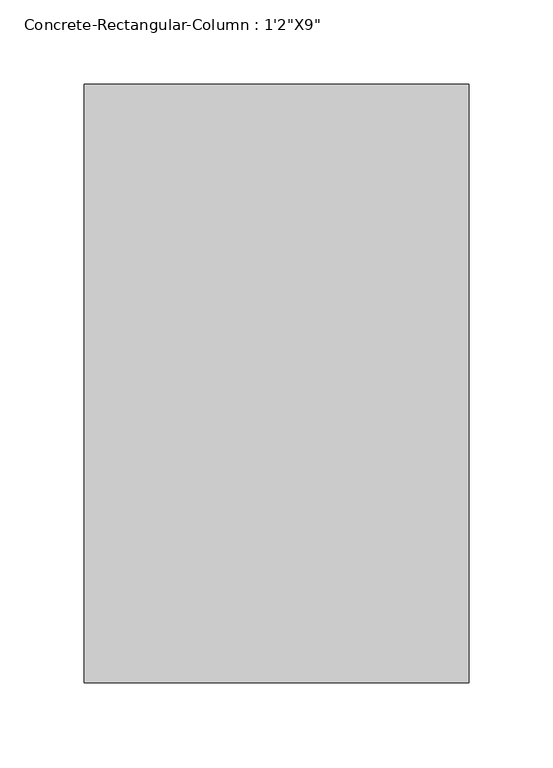
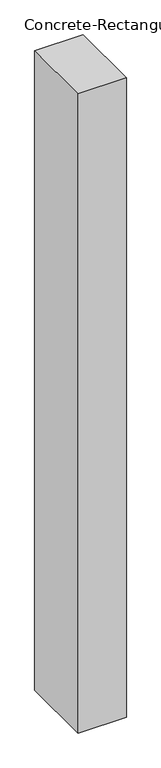
"""IFC4 building model written with IfcOpenShell, lengths in millimetres: column geometry."""

from ifc_helpers import new_model, si_unit, frame, origin, place, context, project, spatial, polyline, outline, extrude, source, transform, mapped, element, save


def column_dd6cc16d(model_context):
    return source(origin(), model_context, "Body", "SweptSolid", [
        extrude(outline(polyline([(114.3, 177.8), (114.3, -177.8), (-114.3, -177.8), (-114.3, 177.8), (114.3, 177.8)])), frame((0.0, 0.0, 16002.0), z_axis=(0.0, 0.0, 1.0), x_axis=(1.0, 0.0, 0.0)), (0.0, 0.0, 1.0), 3200.4),
    ])


if __name__ == "__main__":
    model = new_model("IFC4")
    model_context = context("Model", 3, world=origin())
    ifc_project = project(units=[si_unit("LENGTHUNIT", "METRE", prefix="MILLI")], contexts=[model_context])
    site = spatial("IfcSite", under=ifc_project)
    building = spatial("IfcBuilding", under=site)
    placement = place(None, origin())
    column_shape = column_dd6cc16d(model_context)
    element("IfcColumn", 1, ObjectType="Concrete-Rectangular-Column : 1'2\"X9\"", at=placement, inside=building, context=model_context, shape_type="MappedRepresentation", body=[
        mapped(column_shape, transform((0.0, 0.0, 0.0), x_axis=(1.0, 0.0, 0.0), y_axis=(0.0, 1.0, 0.0), z_axis=(0.0, 0.0, 1.0))),
    ])
    save(model, "model.ifc")

# Revit data of these elements
# Type "Concrete-Rectangular-Column : 1'2\"X9\""
#   Assembly Code = "B10"
#   b = 0' - 9"
#   h = 1' - 2"
#   Structural Material [instance default] = Concrete, Cast-in-Place gray
# Element 1 (IfcColumn, "Concrete-Rectangular-Column : 1'2\"X9\"")
#   Materials on its faces: "Concrete, Cast-in-Place gray"
# Materials
#   "Concrete, Cast-in-Place gray": class "Concrete", colour RGB 192 192 192, transparency 0, Description = "Cast-in-place concrete", Cost = 0
